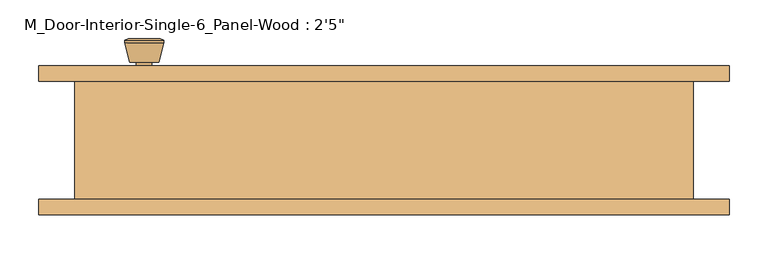
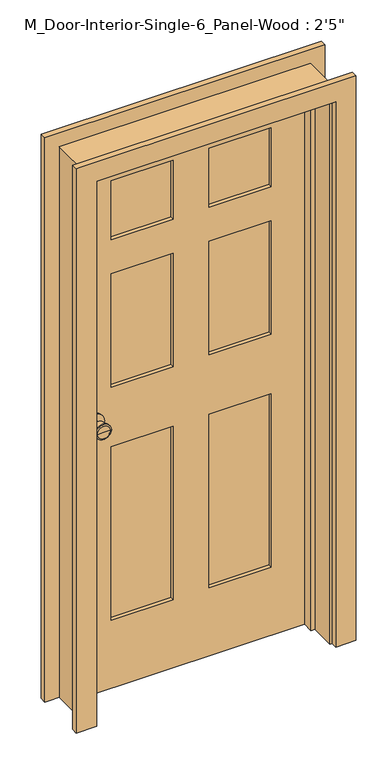
"""IFC4 building model written with IfcOpenShell, lengths in millimetres: door geometry."""

from ifc_helpers import new_model, si_unit, point, frame, frame_2d, origin, place, context, project, spatial, polyline, circle_curve, trimmed, segment, composite_curve, outline, extrude, faceted_brep, source, transform, mapped, element, save
from ifc_brep_helpers import plane_surface, cylinder_surface, revolved_surface, advanced_brep


def door_ef1582a9(model_context):
    return source(origin(), model_context, "Body", "SolidModel", [
        advanced_brep(
        [(-310.0, 32.025, 914.4), (-300.0, 32.025, 914.4), (-320.0, 32.025, 914.4), (-289.5241324, -16.975, 914.4), (-310.0, -16.975, 914.4), (-330.4758676, -16.975, 914.4), (-285.0, -15.1471319, 914.4), (-335.0, -15.1471319, 914.4), (-285.0, -11.6834537, 914.4), (-335.0, -11.6834537, 914.4), (-291.363764, 13.025, 914.4), (-328.636236, 13.025, 914.4), (-300.0, 13.025, 914.4), (-320.0, 13.025, 914.4)],
        [
            (0, 1),
            (1, 2, circle_curve(frame((-310.0, 32.025, 914.4), z_axis=(0.0, 1.0, 0.0), x_axis=(-1.0, 0.0, 0.0)), 10.0)),
            (2, 0),
            (2, 1, circle_curve(frame((-310.0, 32.025, 914.4), z_axis=(0.0, 1.0, 0.0), x_axis=(-1.0, 0.0, 0.0)), 10.0)),
            (3, 4),
            (4, 5),
            (5, 3, circle_curve(frame((-310.0, -16.975, 914.4), z_axis=(0.0, -1.0, 0.0), x_axis=(-1.0, 0.0, 0.0)), 20.4758676)),
            (3, 5, circle_curve(frame((-310.0, -16.975, 914.4), z_axis=(0.0, -1.0, 0.0), x_axis=(-1.0, 0.0, 0.0)), 20.4758676)),
            (6, 3),
            (5, 7),
            (7, 6, circle_curve(frame((-310.0, -15.1471319, 914.4), z_axis=(0.0, -1.0, 0.0), x_axis=(-1.0, 0.0, 0.0)), 25.0)),
            (6, 7, circle_curve(frame((-310.0, -15.1471319, 914.4), z_axis=(0.0, -1.0, 0.0), x_axis=(-1.0, 0.0, 0.0)), 25.0)),
            (8, 6),
            (7, 9),
            (9, 8, circle_curve(frame((-310.0, -11.6834537, 914.4), z_axis=(0.0, -1.0, 0.0), x_axis=(-1.0, 0.0, 0.0)), 25.0)),
            (8, 9, circle_curve(frame((-310.0, -11.6834537, 914.4), z_axis=(0.0, -1.0, 0.0), x_axis=(-1.0, 0.0, 0.0)), 25.0)),
            (10, 8),
            (9, 11),
            (11, 10, circle_curve(frame((-310.0, 13.025, 914.4), z_axis=(0.0, -1.0, 0.0), x_axis=(-1.0, 0.0, 0.0)), 18.636236)),
            (10, 11, circle_curve(frame((-310.0, 13.025, 914.4), z_axis=(0.0, -1.0, 0.0), x_axis=(-1.0, 0.0, 0.0)), 18.636236)),
            (12, 10),
            (11, 13),
            (13, 12, circle_curve(frame((-310.0, 13.025, 914.4), z_axis=(0.0, -1.0, 0.0), x_axis=(-1.0, 0.0, 0.0)), 10.0)),
            (12, 13, circle_curve(frame((-310.0, 13.025, 914.4), z_axis=(0.0, -1.0, 0.0), x_axis=(-1.0, 0.0, 0.0)), 10.0)),
            (1, 12),
            (13, 2),
        ],
        [
            plane_surface(frame((-310.0, 32.025, 914.4), z_axis=(0.0, 1.0, 0.0), x_axis=(-1.0, 0.0, 0.0))),
            plane_surface(frame((-310.0, -16.975, 914.4), z_axis=(0.0, -1.0, 0.0), x_axis=(-1.0, 0.0, 0.0))),
            revolved_surface(polyline([(-330.4758676, -16.975, 914.4), (-335.0, -15.1471319, 914.4)]), (-310.0, 32.025, 914.4), (0.0, 1.0, 0.0)),
            cylinder_surface(frame((-310.0, 32.025, 914.4), z_axis=(0.0, 1.0, 0.0), x_axis=(-1.0, 0.0, 0.0)), 25.0),
            revolved_surface(polyline([(-335.0, -11.6834537, 914.4), (-328.636236, 13.025, 914.4)]), (-310.0, 32.025, 914.4), (0.0, 1.0, 0.0)),
            plane_surface(frame((-310.0, 13.025, 914.4), z_axis=(0.0, 1.0, 0.0), x_axis=(-1.0, 0.0, 0.0))),
            cylinder_surface(frame((-310.0, 32.025, 914.4), z_axis=(0.0, 1.0, 0.0), x_axis=(-1.0, 0.0, 0.0)), 10.0),
        ],
        [
            (0, [[1, 2, 3]]),
            (0, [[-3, 4, -1]]),
            (1, [[5, 6, 7]]),
            (1, [[-6, -5, 8]]),
            (2, [[9, -7, 10, 11]]),
            (2, [[-10, -8, -9, 12]]),
            (3, [[13, -11, 14, 15]]),
            (3, [[-14, -12, -13, 16]]),
            (4, [[17, -15, 18, 19]]),
            (4, [[-18, -16, -17, 20]]),
            (5, [[21, -19, 22, 23]]),
            (5, [[-22, -20, -21, 24]]),
            (6, [[25, -23, 26, -2]]),
            (6, [[-26, -24, -25, -4]]),
        ],
    ),
        extrude(outline(composite_curve([segment(trimmed(circle_curve(frame_2d((914.4, -310.0)), 30.0), [point((914.4, -340.0))], [point((914.4, -280.0))], False, "CARTESIAN"), True, "CONTINUOUS"), segment(trimmed(circle_curve(frame_2d((914.4, -310.0)), 30.0), [point((914.4, -280.0))], [point((914.4, -340.0))], False, "CARTESIAN"), True, "CONTINUOUS")], self_intersect=False)), frame((0.0, 32.025, 0.0), z_axis=(0.0, 1.0, 0.0), x_axis=(0.0, 0.0, 1.0)), (0.0, 0.0, 1.0), 6.0),
        advanced_brep(
        [(-310.0, 79.025, 914.4), (-320.0, 79.025, 914.4), (-300.0, 79.025, 914.4), (-289.5241324, 128.025, 914.4), (-330.4758676, 128.025, 914.4), (-310.0, 128.025, 914.4), (-285.0, 126.1971319, 914.4), (-335.0, 126.1971319, 914.4), (-285.0, 122.7334537, 914.4), (-335.0, 122.7334537, 914.4), (-291.363764, 98.025, 914.4), (-328.636236, 98.025, 914.4), (-300.0, 98.025, 914.4), (-320.0, 98.025, 914.4)],
        [
            (0, 1),
            (1, 2, circle_curve(frame((-310.0, 79.025, 914.4), z_axis=(0.0, -1.0, 0.0), x_axis=(-1.0, 0.0, 0.0)), 10.0)),
            (2, 0),
            (2, 1, circle_curve(frame((-310.0, 79.025, 914.4), z_axis=(0.0, -1.0, 0.0), x_axis=(-1.0, 0.0, 0.0)), 10.0)),
            (3, 4, circle_curve(frame((-310.0, 128.025, 914.4), z_axis=(0.0, 1.0, 0.0), x_axis=(-1.0, 0.0, 0.0)), 20.4758676)),
            (4, 5),
            (5, 3),
            (4, 3, circle_curve(frame((-310.0, 128.025, 914.4), z_axis=(0.0, 1.0, 0.0), x_axis=(-1.0, 0.0, 0.0)), 20.4758676)),
            (6, 7, circle_curve(frame((-310.0, 126.1971319, 914.4), z_axis=(0.0, 1.0, 0.0), x_axis=(-1.0, 0.0, 0.0)), 25.0)),
            (7, 4),
            (3, 6),
            (7, 6, circle_curve(frame((-310.0, 126.1971319, 914.4), z_axis=(0.0, 1.0, 0.0), x_axis=(-1.0, 0.0, 0.0)), 25.0)),
            (8, 9, circle_curve(frame((-310.0, 122.7334537, 914.4), z_axis=(0.0, 1.0, 0.0), x_axis=(-1.0, 0.0, 0.0)), 25.0)),
            (9, 7),
            (6, 8),
            (9, 8, circle_curve(frame((-310.0, 122.7334537, 914.4), z_axis=(0.0, 1.0, 0.0), x_axis=(-1.0, 0.0, 0.0)), 25.0)),
            (10, 11, circle_curve(frame((-310.0, 98.025, 914.4), z_axis=(0.0, 1.0, 0.0), x_axis=(-1.0, 0.0, 0.0)), 18.636236)),
            (11, 9),
            (8, 10),
            (11, 10, circle_curve(frame((-310.0, 98.025, 914.4), z_axis=(0.0, 1.0, 0.0), x_axis=(-1.0, 0.0, 0.0)), 18.636236)),
            (12, 13, circle_curve(frame((-310.0, 98.025, 914.4), z_axis=(0.0, 1.0, 0.0), x_axis=(-1.0, 0.0, 0.0)), 10.0)),
            (13, 11),
            (10, 12),
            (13, 12, circle_curve(frame((-310.0, 98.025, 914.4), z_axis=(0.0, 1.0, 0.0), x_axis=(-1.0, 0.0, 0.0)), 10.0)),
            (1, 13),
            (12, 2),
        ],
        [
            plane_surface(frame((-310.0, 79.025, 914.4), z_axis=(0.0, -1.0, 0.0), x_axis=(-1.0, 0.0, 0.0))),
            plane_surface(frame((-310.0, 128.025, 914.4), z_axis=(0.0, 1.0, 0.0), x_axis=(-1.0, 0.0, 0.0))),
            revolved_surface(polyline([(-330.4758676, 128.025, 914.4), (-335.0, 126.1971319, 914.4)]), (-310.0, 79.025, 914.4), (0.0, -1.0, 0.0)),
            cylinder_surface(frame((-310.0, 79.025, 914.4), z_axis=(0.0, -1.0, 0.0), x_axis=(-1.0, 0.0, 0.0)), 25.0),
            revolved_surface(polyline([(-335.0, 122.7334537, 914.4), (-328.636236, 98.025, 914.4)]), (-310.0, 79.025, 914.4), (0.0, -1.0, 0.0)),
            plane_surface(frame((-310.0, 98.025, 914.4), z_axis=(0.0, -1.0, 0.0), x_axis=(-1.0, 0.0, 0.0))),
            cylinder_surface(frame((-310.0, 79.025, 914.4), z_axis=(0.0, -1.0, 0.0), x_axis=(-1.0, 0.0, 0.0)), 10.0),
        ],
        [
            (0, [[1, 2, 3]]),
            (0, [[-3, 4, -1]]),
            (1, [[5, 6, 7]]),
            (1, [[8, -7, -6]]),
            (2, [[9, 10, -5, 11]]),
            (2, [[12, -11, -8, -10]]),
            (3, [[13, 14, -9, 15]]),
            (3, [[16, -15, -12, -14]]),
            (4, [[17, 18, -13, 19]]),
            (4, [[20, -19, -16, -18]]),
            (5, [[21, 22, -17, 23]]),
            (5, [[24, -23, -20, -22]]),
            (6, [[-2, 25, -21, 26]]),
            (6, [[-4, -26, -24, -25]]),
        ],
    ),
        extrude(outline(composite_curve([segment(trimmed(circle_curve(frame_2d((914.4, -310.0)), 30.0), [point((914.4, -340.0))], [point((914.4, -280.0))], False, "CARTESIAN"), True, "CONTINUOUS"), segment(trimmed(circle_curve(frame_2d((914.4, -310.0)), 30.0), [point((914.4, -280.0))], [point((914.4, -340.0))], False, "CARTESIAN"), True, "CONTINUOUS")], self_intersect=False)), frame((0.0, 73.025, 0.0), z_axis=(0.0, 1.0, 0.0), x_axis=(0.0, 0.0, 1.0)), (0.0, 0.0, 1.0), 6.0),
        faceted_brep([(400.0, 73.025, 0.0), (400.0, -79.375, 0.0), (375.0, -79.375, 0.0), (375.0, 3.1, 0.0), (362.3, 3.1, 0.0), (362.3, 38.025, 0.0), (375.0, 38.025, 0.0), (375.0, 73.025, 0.0), (400.0, 73.025, 1853.8), (400.0, -79.375, 1853.8), (-400.0, -79.375, 1853.8), (-400.0, -79.375, 0.0), (-375.0, -79.375, 0.0), (-375.0, -79.375, 1828.8), (375.0, -79.375, 1828.8), (375.0, 3.1, 1828.8), (-375.0, 3.1, 1828.8), (-375.0, 3.1, 0.0), (-362.3, 3.1, 0.0), (-362.3, 3.1, 1816.1), (362.3, 3.1, 1816.1), (362.3, 38.025, 1816.1), (-362.3, 38.025, 1816.1), (-362.3, 38.025, 0.0), (-375.0, 38.025, 0.0), (-375.0, 38.025, 1828.8), (375.0, 38.025, 1828.8), (375.0, 73.025, 1828.8), (-375.0, 73.025, 1828.8), (-375.0, 73.025, 0.0), (-400.0, 73.025, 0.0), (-400.0, 73.025, 1853.8)], [[[0, 1, 2, 3, 4, 5, 6, 7]], [[1, 0, 8, 9]], [[2, 1, 9, 10, 11, 12, 13, 14]], [[3, 2, 14, 15]], [[4, 3, 15, 16, 17, 18, 19, 20]], [[5, 4, 20, 21]], [[6, 5, 21, 22, 23, 24, 25, 26]], [[7, 6, 26, 27]], [[0, 7, 27, 28, 29, 30, 31, 8]], [[9, 8, 31, 10]], [[15, 14, 13, 16]], [[21, 20, 19, 22]], [[27, 26, 25, 28]], [[30, 29, 24, 23, 18, 17, 12, 11]], [[10, 31, 30, 11]], [[16, 13, 12, 17]], [[22, 19, 18, 23]], [[28, 25, 24, 29]]]),
        extrude(outline(polyline([(1828.8, -375.0), (0.0, -375.0), (0.0, 375.0), (1828.8, 375.0), (1828.8, -375.0)]), holes=[polyline([(1708.8, 57.5), (1708.8, 255.0), (1511.3, 255.0), (1511.3, 57.5), (1708.8, 57.5)]), polyline([(1396.3, 255.0), (1014.4, 255.0), (1014.4, 57.5), (1396.3, 57.5), (1396.3, 255.0)]), polyline([(1014.4, -57.5), (1014.4, -255.0), (1396.3, -255.0), (1396.3, -57.5), (1014.4, -57.5)]), polyline([(1511.3, -255.0), (1708.8, -255.0), (1708.8, -57.5), (1511.3, -57.5), (1511.3, -255.0)]), polyline([(814.4, 57.5), (814.4, 255.0), (230.0, 255.0), (230.0, 57.5), (814.4, 57.5)]), polyline([(230.0, -57.5), (230.0, -255.0), (814.4, -255.0), (814.4, -57.5), (230.0, -57.5)])]), frame((0.0, 38.025, 0.0), z_axis=(0.0, 1.0, 0.0), x_axis=(0.0, 0.0, 1.0)), (0.0, 0.0, 1.0), 35.0),
        extrude(outline(polyline([(255.0, 49.6916667), (57.5, 49.6916667), (57.5, 61.3583333), (255.0, 61.3583333), (255.0, 49.6916667)])), frame((0.0, 0.0, 1511.3), z_axis=(0.0, 0.0, 1.0), x_axis=(1.0, 0.0, 0.0)), (0.0, 0.0, 1.0), 197.5),
        extrude(outline(polyline([(255.0, 49.6916667), (57.5, 49.6916667), (57.5, 61.3583333), (255.0, 61.3583333), (255.0, 49.6916667)])), frame((0.0, 0.0, 1014.4), z_axis=(0.0, 0.0, 1.0), x_axis=(1.0, 0.0, 0.0)), (0.0, 0.0, 1.0), 381.9),
        extrude(outline(polyline([(-57.5, 49.6916667), (-255.0, 49.6916667), (-255.0, 61.3583333), (-57.5, 61.3583333), (-57.5, 49.6916667)])), frame((0.0, 0.0, 1014.4), z_axis=(0.0, 0.0, 1.0), x_axis=(1.0, 0.0, 0.0)), (0.0, 0.0, 1.0), 381.9),
        extrude(outline(polyline([(-57.5, 49.6916667), (-255.0, 49.6916667), (-255.0, 61.3583333), (-57.5, 61.3583333), (-57.5, 49.6916667)])), frame((0.0, 0.0, 1511.3), z_axis=(0.0, 0.0, 1.0), x_axis=(1.0, 0.0, 0.0)), (0.0, 0.0, 1.0), 197.5),
        extrude(outline(polyline([(255.0, 49.6916667), (57.5, 49.6916667), (57.5, 61.3583333), (255.0, 61.3583333), (255.0, 49.6916667)])), frame((0.0, 0.0, 230.0), z_axis=(0.0, 0.0, 1.0), x_axis=(1.0, 0.0, 0.0)), (0.0, 0.0, 1.0), 584.4),
        extrude(outline(polyline([(-57.5, 49.6916667), (-255.0, 49.6916667), (-255.0, 61.3583333), (-57.5, 61.3583333), (-57.5, 49.6916667)])), frame((0.0, 0.0, 230.0), z_axis=(0.0, 0.0, 1.0), x_axis=(1.0, 0.0, 0.0)), (0.0, 0.0, 1.0), 584.4),
        extrude(outline(polyline([(0.0, 381.35), (0.0, 446.35), (1900.15, 446.35), (1900.15, -446.35), (0.0, -446.35), (0.0, -381.35), (1835.15, -381.35), (1835.15, 381.35), (0.0, 381.35)])), frame((0.0, 73.025, 0.0), z_axis=(0.0, 1.0, 0.0), x_axis=(0.0, 0.0, 1.0)), (0.0, 0.0, 1.0), 20.0),
        extrude(outline(polyline([(0.0, 381.35), (0.0, 446.35), (1900.15, 446.35), (1900.15, -446.35), (0.0, -446.35), (0.0, -381.35), (1835.15, -381.35), (1835.15, 381.35), (0.0, 381.35)])), frame((0.0, -99.375, 0.0), z_axis=(0.0, 1.0, 0.0), x_axis=(0.0, 0.0, 1.0)), (0.0, 0.0, 1.0), 20.0),
    ])


if __name__ == "__main__":
    model = new_model("IFC4")
    model_context = context("Model", 3, world=origin())
    ifc_project = project(units=[si_unit("LENGTHUNIT", "METRE", prefix="MILLI")], contexts=[model_context])
    site = spatial("IfcSite", under=ifc_project)
    building = spatial("IfcBuilding", under=site)
    placement = place(None, origin())
    door_shape = door_ef1582a9(model_context)
    element("IfcDoor", 1, ObjectType="M_Door-Interior-Single-6_Panel-Wood : 2'5\"", at=placement, inside=building, context=model_context, shape_type="MappedRepresentation", body=[
        mapped(door_shape, transform((0.0, 0.0, 0.0), x_axis=(1.0, 0.0, 0.0), y_axis=(0.0, 1.0, 0.0), z_axis=(0.0, 0.0, 1.0))),
    ])
    save(model, "model.ifc")

# Revit data of these elements
# Type "M_Door-Interior-Single-6_Panel-Wood : 2'5\""
#   Type Mark = "11"
#   Assembly Code = "C1020300"
#   Analytic Construction = "Wooden"
#   Top Rail = 0' - 4.72441"
#   Top Panel = 0' - 7.77559"
#   Thickness = 0' - 1.37795"
#   Thermal Resistance (R) = 2.5876 (h·ft²·°F)/BTU
#   Swing Angle [instance default] = 90.00°
#   Stiles = 0' - 4.72441"
#   Rough Width = 2' - 7.49606"
#   Rough Height = 6' - 0.98425"
#   Mullion = 0' - 4.52756"
#   Lock Rail = 0' - 7.87402"
#   Intermediate Rail = 0' - 4.52756"
#   Height = 6' - 0"
#   Width = 2' - 5.52756"
#   Heat Transfer Coefficient (U) = 0.3865 BTU/(h·ft²·°F)
#   Bottom Rail = 0' - 9.05512"
#   Trim Material = Cherry
#   Panel Material = Cherry
#   Frame Material = Cherry
#   Door Handle Material = Aluminum
#   Visual Light Transmittance = 0
#   Solar Heat Gain Coefficient = 0
#   Wall Closure = (empty or 0)
#   Function = (empty or 0)
# Element 1 (IfcDoor, "M_Door-Interior-Single-6_Panel-Wood : 2'5\"")
#   Materials on its faces: "Cherry", "Aluminum"
# Materials
#   "Cherry": class "Wood", colour RGB 226 177 128, transparency 0, Description = "Prunus Serotina", Cost = 0
#   "Aluminum": class "Metal", colour RGB 247 247 247, transparency 0, Description = "Aluminum 6061", Cost = 0
